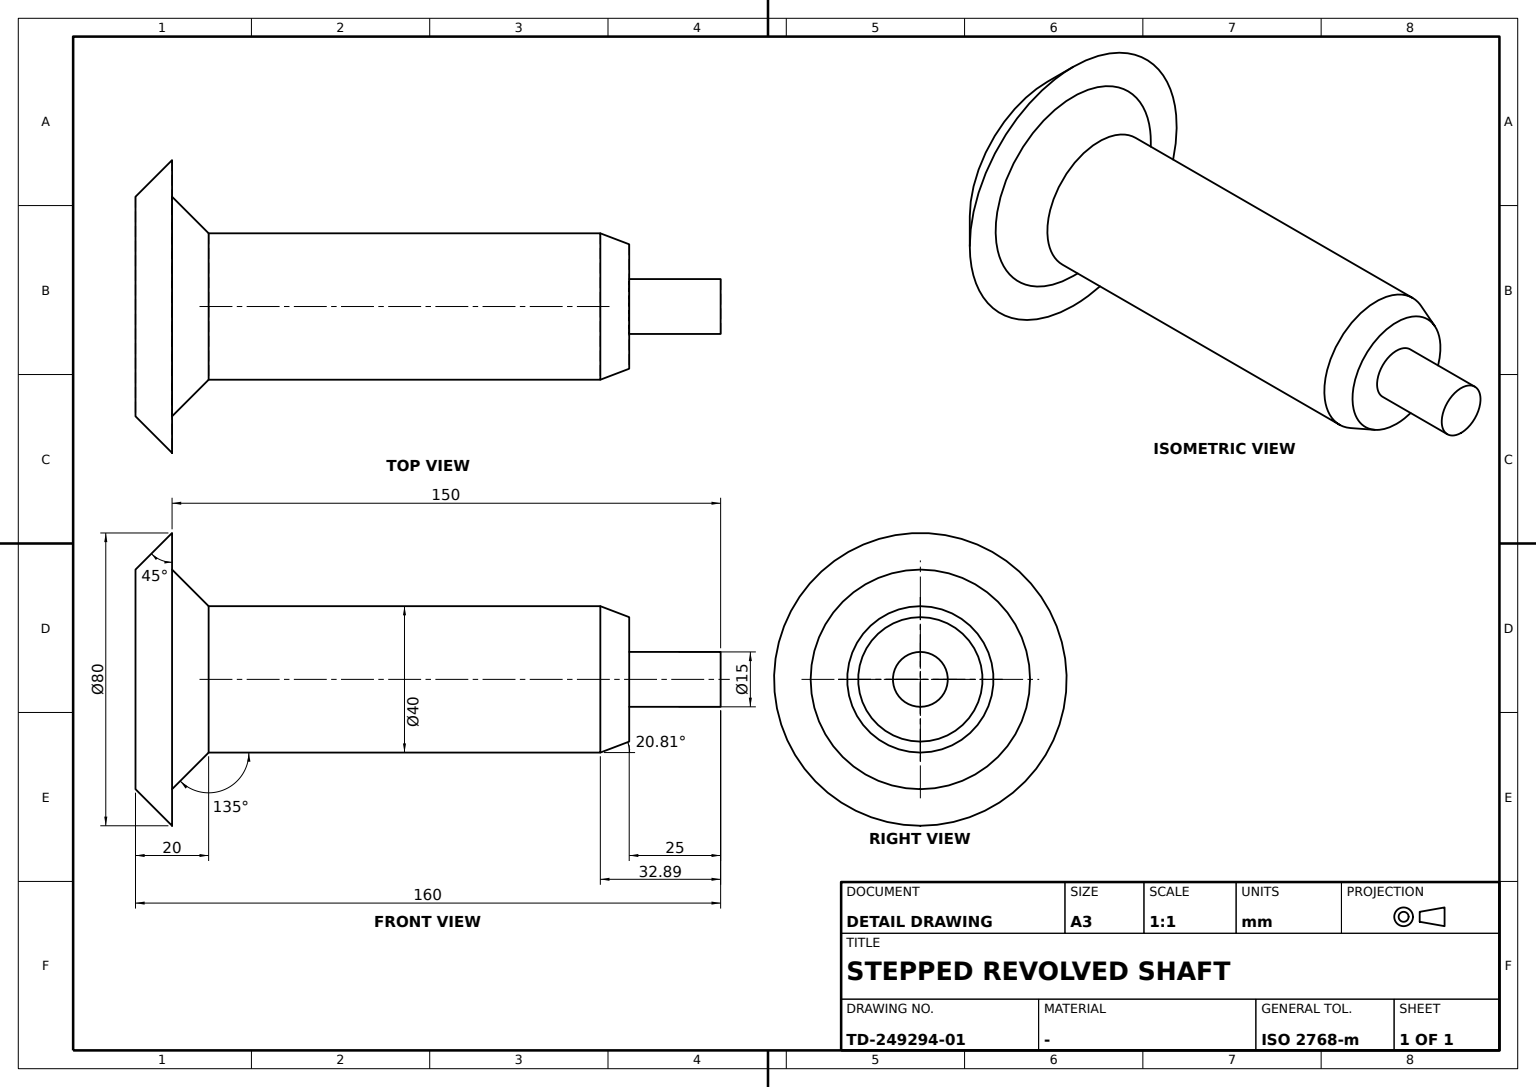
CATIA V5 part; units mm, degrees
sketch "Sketch1" plane through (0, 0, 0) normal (-1, 0, 0) x (0, -1, 0)
  line L0 (0, 0) -> (0, 7.5)
  point P0 (0, 7.5)
  line L1 (0, 7.5) -> (25, 7.5)
  line L2 (25, 7.5) -> (25, 17)
  line L3 (25, 17) -> (32.8947, 20)
  line L4 (32.8947, 20) -> (150, 20)
  point P1 (150, 20)
  point P2 (150, 20)
  line L5 (150, 20) -> (150, 40)
  point P3 (150, 40)
  line L6 (150, 40) -> (160, 40)
  line L7 (160, 40) -> (160, 0)
  point P4 (160, 0)
  line L8 (0, 0) -> (160, 0)
  dimension "length L0" = 7.5
  dimension "length L3 y axis" = 3
  dimension "length L1" = 25
  dimension "distance L8 L4" = 20
  dimension "distance y axis P3" = 150
  dimension "distance L6 L8" = 40
  dimension "length L6" = 10
  constraint vertical L0 y-axis
  constraint vertical L2 y-axis
  constraint vertical L5 y-axis
  constraint vertical L7 y-axis
  constraint horizontal L1 x-axis
  constraint horizontal L4 x-axis
  constraint horizontal L8 x-axis
  constraint coincidence L3 P0
  constraint coincidence P4 x-axis
  constraint coincidence P1 P2
revolve "Shaft1" add sketch "Sketch1" angle 360 about L8
chamfer "Chamfer1" distance 10 angle 45 1 edges at (0, -150, -20)
chamfer "Chamfer2" distance 10 angle 45 1 edges at (0, -160, -40)
